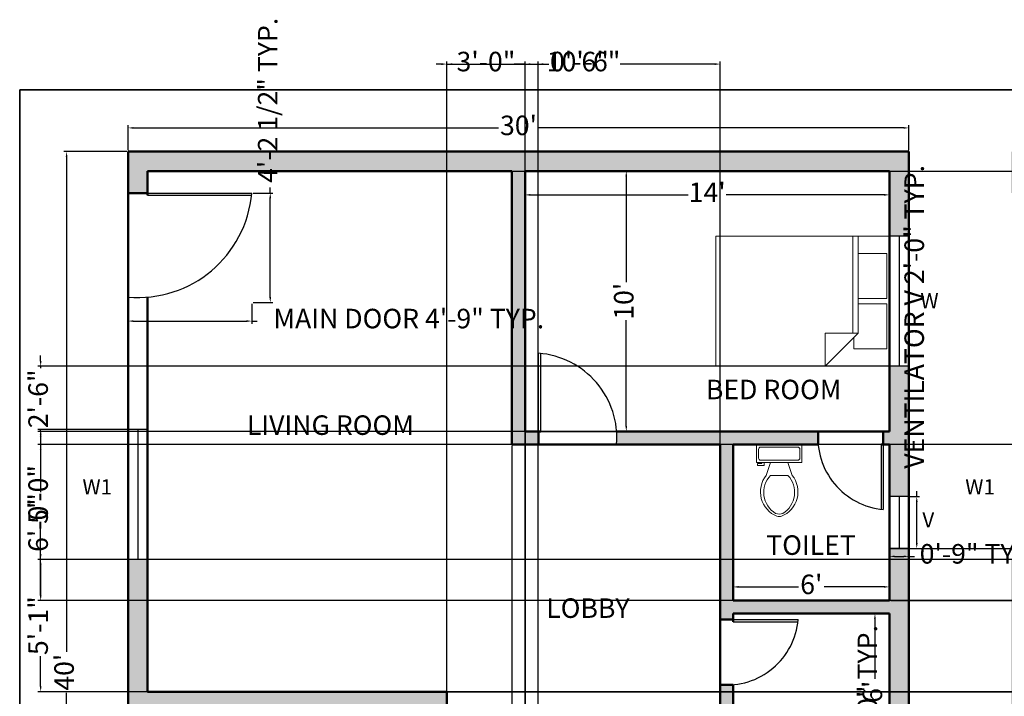
# Model space of a CAD drawing. Units: inches. Extents: x 2463 to 3327, y 6994 to 7582.
# Tile 3 of 5: x 2463 to 2917, y 7270 to 7582. Entities that reach past the tile are written whole.
import ezdxf

# ---------------------------------------------------------------- set-up
doc = ezdxf.new("R2010")
doc.units = ezdxf.units.IN
for name, color, linetype, lineweight in [('A-ANNO-DIMS', 2, 'Continuous', 18), ('A-ANNO-TEXT', 7, 'Continuous', 18), ('A-ANNO-TTLB', 7, 'Continuous', 35), ('A-AREA-IDEN', 3, 'Continuous', 25), ('A-DOOR', 4, 'Continuous', 25), ('A-FLOR-FIXT', 8, 'Continuous', 18), ('A-FURN', 8, 'Continuous', 18), ('A-GLAZ', 4, 'Continuous', 25), ('A-WALL', 7, 'Continuous', 50), ('A-WALL-PATT', 252, 'Continuous', 13)]:
    doc.layers.add(name, color=color, linetype=linetype, lineweight=lineweight)
doc.styles.get("Standard").update_dxf_attribs({"font": 'times.ttf'})
doc.dimstyles.new('ISO-25', dxfattribs={"dimtxt": 9, "dimasz": 2.5, "dimexe": 1.25, "dimexo": 0.625, "dimgap": 2, "dimtad": 0, "dimdec": 1, "dimlunit": 4, "dimtxsty": 'Standard', "dimcen": 2.5, "dimadec": 0, "dimazin": 0, "dimtfac": 1, "dimtdec": 1, "dimtmove": 0, "dimatfit": 3, "dimfxl": 1, "dimarcsym": 0})

# ---------------------------------------------------------------- blocks, each defined once
blk = doc.blocks.new('*D1')
at = {"layer": 'A-ANNO-DIMS', "color": 0, "lineweight": -2, "transparency": 16777216}
for p, q in [((2696.43, 7511.2), (2696.43, 7499.6)), ((2864.43, 7511.2), (2864.43, 7499.6)), ((2698.93, 7500.85), (2771.65, 7500.85)), ((2861.93, 7500.85), (2789.21, 7500.85))]:
    blk.add_line(p, q, dxfattribs=at)
at = {"layer": 'A-ANNO-DIMS', "color": 0, "transparency": 16777216}
for points in [[(2698.93, 7501.27), (2698.93, 7500.43), (2696.43, 7500.85)], [(2861.93, 7501.27), (2861.93, 7500.43), (2864.43, 7500.85)]]:
    blk.add_solid(points, dxfattribs=at)
at = {"layer": 'Defpoints', "color": 0, "transparency": 16777216}
for p in [(2696.43, 7511.83), (2864.43, 7511.83), (2864.43, 7500.85)]:
    blk.add_point(p, dxfattribs=at)
at = {"layer": 'A-ANNO-DIMS', "color": 0, "transparency": 16777216, "insert": (2780.43, 7500.85), "char_height": 9, "attachment_point": 5}
blk.add_mtext("14'", dxfattribs=at)
blk = doc.blocks.new('*D2')
at = {"layer": 'A-ANNO-DIMS', "color": 0, "lineweight": -2, "transparency": 16777216}
for p, q in [((2697.06, 7511.83), (2744.37, 7511.83)), ((2743.12, 7509.33), (2743.12, 7460.61)), ((2743.12, 7394.33), (2743.12, 7443.04)), ((2697.06, 7391.83), (2744.37, 7391.83))]:
    blk.add_line(p, q, dxfattribs=at)
at = {"layer": 'A-ANNO-DIMS', "color": 0, "transparency": 16777216}
for points in [[(2742.7, 7509.33), (2743.53, 7509.33), (2743.12, 7511.83)], [(2742.7, 7394.33), (2743.53, 7394.33), (2743.12, 7391.83)]]:
    blk.add_solid(points, dxfattribs=at)
at = {"layer": 'Defpoints', "color": 0, "transparency": 16777216}
for p in [(2696.43, 7511.83), (2696.43, 7391.83), (2743.12, 7391.83)]:
    blk.add_point(p, dxfattribs=at)
at = {"layer": 'A-ANNO-DIMS', "color": 0, "transparency": 16777216, "insert": (2743.12, 7451.83), "char_height": 9, "attachment_point": 5, "rotation": 90}
blk.add_mtext("10'", dxfattribs=at)
blk = doc.blocks.new('*D3')
at = {"layer": 'A-ANNO-DIMS', "color": 0, "lineweight": -2, "transparency": 16777216}
for p, q in [((2863.81, 7307.83), (2856.5, 7307.83)), ((2857.75, 7305.33), (2857.75, 7277.78)), ((2857.75, 7238.33), (2857.75, 7265.87)), ((2863.81, 7235.83), (2856.5, 7235.83))]:
    blk.add_line(p, q, dxfattribs=at)
at = {"layer": 'A-ANNO-DIMS', "color": 0, "transparency": 16777216}
for points in [[(2857.34, 7305.33), (2858.17, 7305.33), (2857.75, 7307.83)], [(2857.34, 7238.33), (2858.17, 7238.33), (2857.75, 7235.83)]]:
    blk.add_solid(points, dxfattribs=at)
at = {"layer": 'Defpoints', "color": 0, "transparency": 16777216}
for p in [(2857.75, 7307.83), (2864.43, 7307.83), (2864.43, 7235.83)]:
    blk.add_point(p, dxfattribs=at)
at = {"layer": 'A-ANNO-DIMS', "color": 0, "transparency": 16777216, "insert": (2857.75, 7271.83), "char_height": 9, "attachment_point": 5, "rotation": 90}
blk.add_mtext("6'", dxfattribs=at)
blk = doc.blocks.new('Bed - Queen')
for p, q in [((0, -80.00003), (0, 0)), ((0, 0), (59.99999, 0)), ((59.99999, 0), (59.99999, -80.00003)), ((7.99999, -1.2), (28.79998, -1.2)), ((7.99999, -14.4), (7.99999, -1.2)), ((28.79998, -1.2), (28.79998, -14.4)), ((31.19999, -1.2), (51.99999, -1.2)), ((31.19999, -14.4), (31.19999, -1.2)), ((51.99999, -1.2), (51.99999, -16.4)), ((0, -14.4), (44.8, -14.4)), ((44.8, -16.8), (0, -16.8)), ((59.99999, -29.6), (44.8, -14.4)), ((44.8, -14.4), (44.8, -29.6)), ((51.99999, -16.4), (46.79936, -16.4)), ((44.8, -29.6), (59.99999, -29.6)), ((59.99999, -80.00003), (0, -80.00003))]:
    blk.add_line(p, q)
blk = doc.blocks.new('*D13')
at = {"layer": 'A-ANNO-DIMS', "color": 0, "lineweight": -2, "transparency": 16777216}
for p, q in [((2792.43, 7314.45), (2792.43, 7321.4)), ((2794.93, 7320.15), (2822.48, 7320.15)), ((2861.93, 7320.15), (2834.38, 7320.15)), ((2864.43, 7314.45), (2864.43, 7321.4))]:
    blk.add_line(p, q, dxfattribs=at)
at = {"layer": 'A-ANNO-DIMS', "color": 0, "transparency": 16777216}
for points in [[(2794.93, 7320.57), (2794.93, 7319.73), (2792.43, 7320.15)], [(2861.93, 7320.57), (2861.93, 7319.73), (2864.43, 7320.15)]]:
    blk.add_solid(points, dxfattribs=at)
at = {"layer": 'Defpoints', "color": 0, "transparency": 16777216}
for p in [(2864.43, 7320.15), (2792.43, 7313.83), (2864.43, 7313.83)]:
    blk.add_point(p, dxfattribs=at)
at = {"layer": 'A-ANNO-DIMS', "color": 0, "transparency": 16777216, "insert": (2828.43, 7320.15), "char_height": 9, "attachment_point": 5}
blk.add_mtext("6'", dxfattribs=at)
blk = doc.blocks.new('*U11')
for p, q in [((9.5, -6), (9.5, -2)), ((-10, -8.5), (-8, -8.5)), ((-10, -9.5), (-10, -8.5)), ((-8, -8.5), (-8, -8)), ((-7, -8), (-7, -9.5)), ((-4, -8), (-6, -14)), ((4, -8), (6, -14)), ((-7, -9.5), (-10, -9.5)), ((4, -14), (-4, -14))]:
    blk.add_line(p, q)
blk.add_lwpolyline([(10.5, -8), (10.5, 0), (-10.5, 0), (-10.5, -8)], close=True)
for points in [[(-9.5, -2), (-9.5, -6)], [(8.5, -1), (-8.5, -1)], [(-8.5, -7), (8.5, -7)]]:
    blk.add_lwpolyline(points)
for centre, radius, start, end in [((-8.62, -1.88), 0.884, 81.8699, 188.1301), ((8.62, -1.88), 0.884, 351.8699, 98.1301), ((-8.62, -6.12), 0.884, 171.8699, 278.1301), ((8.62, -6.12), 0.884, 261.8699, 8.1301), ((3.52, -21.58), 12.17, 141.4691, 247.9714), ((4.2, -21.82), 11.33, 136.3677, 238.9468), ((-3.52, -21.58), 12.17, 292.0284, 38.5307), ((-4.2, -21.82), 11.33, 301.053, 43.6321), ((0, -27.88), 4, 245.7318, 294.2682), ((0, -29), 4, 254.8605, 285.1395)]:
    blk.add_arc(centre, radius, start, end)
blk = doc.blocks.new('*D24')
at = {"layer": 'A-ANNO-DIMS', "color": 0, "lineweight": -2, "transparency": 16777216}
for p, q in [((2513.43, 7521.45), (2513.43, 7532.96)), ((2515.93, 7531.71), (2684.14, 7531.71)), ((2870.93, 7531.71), (2702.72, 7531.71)), ((2873.43, 7521.45), (2873.43, 7532.96))]:
    blk.add_line(p, q, dxfattribs=at)
at = {"layer": 'A-ANNO-DIMS', "color": 0, "transparency": 16777216}
for points in [[(2515.93, 7532.13), (2515.93, 7531.29), (2513.43, 7531.71)], [(2870.93, 7532.13), (2870.93, 7531.29), (2873.43, 7531.71)]]:
    blk.add_solid(points, dxfattribs=at)
at = {"layer": 'Defpoints', "color": 0, "transparency": 16777216}
for p in [(2873.43, 7531.71), (2513.43, 7520.83), (2873.43, 7520.83)]:
    blk.add_point(p, dxfattribs=at)
at = {"layer": 'A-ANNO-DIMS', "color": 0, "transparency": 16777216, "insert": (2693.43, 7531.71), "char_height": 9, "attachment_point": 5}
blk.add_mtext("30'", dxfattribs=at)
blk = doc.blocks.new('*D26')
at = {"layer": 'A-ANNO-DIMS', "color": 0, "lineweight": -2, "transparency": 16777216}
for p, q in [((2512.81, 7520.83), (2483.85, 7520.83)), ((2485.1, 7518.33), (2485.1, 7290.28)), ((2485.1, 7043.33), (2485.1, 7271.37)), ((2512.81, 7040.83), (2483.85, 7040.83))]:
    blk.add_line(p, q, dxfattribs=at)
at = {"layer": 'A-ANNO-DIMS', "color": 0, "transparency": 16777216}
for points in [[(2484.68, 7518.33), (2485.51, 7518.33), (2485.1, 7520.83)], [(2484.68, 7043.33), (2485.51, 7043.33), (2485.1, 7040.83)]]:
    blk.add_solid(points, dxfattribs=at)
at = {"layer": 'Defpoints', "color": 0, "transparency": 16777216}
for p in [(2513.43, 7520.83), (2485.1, 7040.83), (2513.43, 7040.83)]:
    blk.add_point(p, dxfattribs=at)
at = {"layer": 'A-ANNO-DIMS', "color": 0, "transparency": 16777216, "insert": (2485.1, 7280.83), "char_height": 9, "attachment_point": 5, "rotation": 90}
blk.add_mtext("40'", dxfattribs=at)
blk = doc.blocks.new('DOOR-36')
for p, q in [((0, 6), (0, 42)), ((1, 6), (1, 41.91))]:
    blk.add_line(p, q)
blk.add_arc((-3, 3), 39.12, 355.6013, 85.6013)
blk = doc.blocks.new('DOOR-30')
for p, q in [((29.14, 30), (29.14, 0)), ((30.14, 30), (30.14, 0))]:
    blk.add_line(p, q)
blk.add_arc((33.14, 33), 33.14, 174.8056, 264.8056)
blk = doc.blocks.new('DOOR-48')
for p, q in [((9, 48.19), (57, 48.19)), ((9, 47.19), (56.91, 47.19))]:
    blk.add_line(p, q)
blk.add_arc((4.5, 52.69), 52.69, 265.1009, 355.1009)
blk = doc.blocks.new('WIN-60')
for p, q in [((9, 60), (0, 60)), ((4.5, 60), (4.5, 0)), ((9, 0), (0, 0))]:
    blk.add_line(p, q)
blk = doc.blocks.new('WIN-24')
for p, q in [((9, 24), (0, 24)), ((4.5, 24), (4.5, 0)), ((9, 0), (0, 0))]:
    blk.add_line(p, q)
blk = doc.blocks.new('*D37')
at = {"layer": 'A-ANNO-DIMS', "color": 0, "lineweight": -2, "transparency": 16777216}
for p, q in [((2855.43, 7169.83), (2855.43, 7172.33)), ((2863.81, 7169.83), (2854.18, 7169.83)), ((2855.43, 7112.33), (2855.43, 7167.33)), ((2863.81, 7109.83), (2854.18, 7109.83))]:
    blk.add_line(p, q, dxfattribs=at)
at = {"layer": 'A-ANNO-DIMS', "color": 0, "transparency": 16777216}
for points in [[(2855.01, 7167.33), (2855.85, 7167.33), (2855.43, 7169.83)], [(2855.01, 7112.33), (2855.85, 7112.33), (2855.43, 7109.83)]]:
    blk.add_solid(points, dxfattribs=at)
at = {"layer": 'Defpoints', "color": 0, "transparency": 16777216}
for p in [(2855.43, 7169.83), (2864.43, 7169.83), (2864.43, 7109.83)]:
    blk.add_point(p, dxfattribs=at)
at = {"layer": 'A-ANNO-DIMS', "color": 0, "transparency": 16777216, "insert": (2855.43, 7241.15), "char_height": 9, "attachment_point": 5, "rotation": 90}
blk.add_mtext('WINDOW W 5\'-0" TYP.', dxfattribs=at)
blk = doc.blocks.new('*D39')
at = {"layer": 'A-ANNO-DIMS', "color": 0, "lineweight": -2, "transparency": 16777216}
for p, q in [((2877.03, 7361.83), (2877.03, 7364.33)), ((2874.06, 7361.83), (2878.28, 7361.83)), ((2877.03, 7340.33), (2877.03, 7359.33)), ((2874.06, 7337.83), (2878.28, 7337.83))]:
    blk.add_line(p, q, dxfattribs=at)
at = {"layer": 'A-ANNO-DIMS', "color": 0, "transparency": 16777216}
for points in [[(2876.61, 7359.33), (2877.45, 7359.33), (2877.03, 7361.83)], [(2876.61, 7340.33), (2877.45, 7340.33), (2877.03, 7337.83)]]:
    blk.add_solid(points, dxfattribs=at)
at = {"layer": 'Defpoints', "color": 0, "transparency": 16777216}
for p in [(2873.43, 7361.83), (2877.03, 7361.83), (2873.43, 7337.83)]:
    blk.add_point(p, dxfattribs=at)
at = {"layer": 'A-ANNO-DIMS', "color": 0, "transparency": 16777216, "insert": (2877.03, 7444.63), "char_height": 9, "attachment_point": 5, "rotation": 90}
blk.add_mtext('VENTILATOR V 2\'-0" TYP.', dxfattribs=at)
blk = doc.blocks.new('*D40')
at = {"layer": 'A-ANNO-DIMS', "color": 0, "lineweight": -2, "transparency": 16777216}
for p, q in [((2864.43, 7337.2), (2864.43, 7332.98)), ((2873.43, 7337.2), (2873.43, 7332.98)), ((2866.93, 7334.23), (2870.93, 7334.23)), ((2873.43, 7334.23), (2875.93, 7334.23))]:
    blk.add_line(p, q, dxfattribs=at)
at = {"layer": 'A-ANNO-DIMS', "color": 0, "transparency": 16777216}
for points in [[(2866.93, 7334.64), (2866.93, 7333.81), (2864.43, 7334.23)], [(2870.93, 7334.64), (2870.93, 7333.81), (2873.43, 7334.23)]]:
    blk.add_solid(points, dxfattribs=at)
at = {"layer": 'Defpoints', "color": 0, "transparency": 16777216}
for p in [(2864.43, 7337.83), (2873.43, 7337.83), (2873.43, 7334.23)]:
    blk.add_point(p, dxfattribs=at)
at = {"layer": 'A-ANNO-DIMS', "color": 0, "transparency": 16777216, "insert": (2905.86, 7334.23), "char_height": 9, "attachment_point": 5}
blk.add_mtext('0\'-9" TYP.', dxfattribs=at)
blk = doc.blocks.new('*D47')
at = {"layer": 'A-ANNO-DIMS', "color": 0, "lineweight": -2, "transparency": 16777216}
for p, q in [((2513.43, 7450.6), (2513.43, 7441.42)), ((2570.43, 7450.6), (2570.43, 7441.42)), ((2515.93, 7442.67), (2567.93, 7442.67)), ((2570.43, 7442.67), (2572.93, 7442.67))]:
    blk.add_line(p, q, dxfattribs=at)
at = {"layer": 'A-ANNO-DIMS', "color": 0, "transparency": 16777216}
for points in [[(2515.93, 7443.09), (2515.93, 7442.26), (2513.43, 7442.67)], [(2567.93, 7443.09), (2567.93, 7442.26), (2570.43, 7442.67)]]:
    blk.add_solid(points, dxfattribs=at)
at = {"layer": 'Defpoints', "color": 0, "transparency": 16777216}
for p in [(2513.43, 7451.22), (2570.43, 7451.22), (2570.43, 7442.67)]:
    blk.add_point(p, dxfattribs=at)
at = {"layer": 'A-ANNO-DIMS', "color": 0, "transparency": 16777216, "insert": (2642.86, 7442.67), "char_height": 9, "attachment_point": 5}
blk.add_mtext('MAIN DOOR 4\'-9" TYP.', dxfattribs=at)
blk = doc.blocks.new('*D48')
at = {"layer": 'A-ANNO-DIMS', "color": 0, "lineweight": -2, "transparency": 16777216}
for p, q in [((2578.98, 7501.71), (2578.98, 7504.21)), ((2571.06, 7501.71), (2580.23, 7501.71)), ((2578.98, 7453.72), (2578.98, 7499.21)), ((2571.06, 7451.22), (2580.23, 7451.22))]:
    blk.add_line(p, q, dxfattribs=at)
at = {"layer": 'A-ANNO-DIMS', "color": 0, "transparency": 16777216}
for points in [[(2578.56, 7499.21), (2579.4, 7499.21), (2578.98, 7501.71)], [(2578.56, 7453.72), (2579.4, 7453.72), (2578.98, 7451.22)]]:
    blk.add_solid(points, dxfattribs=at)
at = {"layer": 'Defpoints', "color": 0, "transparency": 16777216}
for p in [(2570.43, 7501.71), (2578.98, 7501.71), (2570.43, 7451.22)]:
    blk.add_point(p, dxfattribs=at)
at = {"layer": 'A-ANNO-DIMS', "color": 0, "transparency": 16777216, "insert": (2578.98, 7544.43), "char_height": 9, "attachment_point": 5, "rotation": 90}
blk.add_mtext('4\'-2 1/2" TYP.', dxfattribs=at)
blk = doc.blocks.new('*D49')
at = {"layer": 'A-ANNO-DIMS', "color": 0, "lineweight": -2, "transparency": 16777216}
for p, q in [((2696.43, 7391.2), (2696.43, 6999.28)), ((2690.43, 7385.2), (2690.43, 6999.28)), ((2687.93, 7000.53), (2685.43, 7000.53)), ((2690.43, 7000.53), (2696.43, 7000.53)), ((2698.93, 7000.53), (2701.43, 7000.53))]:
    blk.add_line(p, q, dxfattribs=at)
at = {"layer": 'A-ANNO-DIMS', "color": 0, "transparency": 16777216}
for points in [[(2687.93, 7000.94), (2687.93, 7000.11), (2690.43, 7000.53)], [(2698.93, 7000.94), (2698.93, 7000.11), (2696.43, 7000.53)]]:
    blk.add_solid(points, dxfattribs=at)
at = {"layer": 'Defpoints', "color": 0, "transparency": 16777216}
for p in [(2696.43, 7391.83), (2690.43, 7385.83), (2696.43, 7000.53)]:
    blk.add_point(p, dxfattribs=at)
at = {"layer": 'A-ANNO-DIMS', "color": 0, "transparency": 16777216, "insert": (2715.52, 7000.53), "char_height": 9, "attachment_point": 5}
blk.add_mtext('0\'-6"', dxfattribs=at)
blk = doc.blocks.new('*D50')
at = {"layer": 'A-ANNO-DIMS', "color": 0, "lineweight": -2, "transparency": 16777216}
for p, q in [((2791.81, 7385.83), (2471.88, 7385.83)), ((2473.13, 7383.33), (2473.13, 7363.87)), ((2473.13, 7316.33), (2473.13, 7335.79)), ((2791.81, 7313.83), (2471.88, 7313.83))]:
    blk.add_line(p, q, dxfattribs=at)
at = {"layer": 'A-ANNO-DIMS', "color": 0, "transparency": 16777216}
for points in [[(2472.71, 7383.33), (2473.55, 7383.33), (2473.13, 7385.83)], [(2472.71, 7316.33), (2473.55, 7316.33), (2473.13, 7313.83)]]:
    blk.add_solid(points, dxfattribs=at)
at = {"layer": 'Defpoints', "color": 0, "transparency": 16777216}
for p in [(2792.43, 7385.83), (2473.13, 7313.83), (2792.43, 7313.83)]:
    blk.add_point(p, dxfattribs=at)
at = {"layer": 'A-ANNO-DIMS', "color": 0, "transparency": 16777216, "insert": (2473.13, 7349.83), "char_height": 9, "attachment_point": 5, "rotation": 90}
blk.add_mtext('6\'-0"', dxfattribs=at)
blk = doc.blocks.new('*D51')
at = {"layer": 'A-ANNO-DIMS', "color": 0, "lineweight": -2, "transparency": 16777216}
for p, q in [((2523.06, 7511.83), (3321.97, 7511.83)), ((3320.72, 7509.33), (3320.72, 7409.33)), ((3320.72, 7274.33), (3320.72, 7374.32)), ((2523.06, 7271.83), (3321.97, 7271.83))]:
    blk.add_line(p, q, dxfattribs=at)
at = {"layer": 'A-ANNO-DIMS', "color": 0, "transparency": 16777216}
for points in [[(3320.31, 7509.33), (3321.14, 7509.33), (3320.72, 7511.83)], [(3320.31, 7274.33), (3321.14, 7274.33), (3320.72, 7271.83)]]:
    blk.add_solid(points, dxfattribs=at)
at = {"layer": 'Defpoints', "color": 0, "transparency": 16777216}
for p in [(2522.43, 7511.83), (2522.43, 7271.83), (3320.72, 7271.83)]:
    blk.add_point(p, dxfattribs=at)
at = {"layer": 'A-ANNO-DIMS', "color": 0, "transparency": 16777216, "insert": (3320.72, 7391.83), "char_height": 9, "attachment_point": 5, "rotation": 90}
blk.add_mtext('20\'-0"', dxfattribs=at)
blk = doc.blocks.new('*D52')
at = {"layer": 'A-ANNO-DIMS', "color": 0, "lineweight": -2, "transparency": 16777216}
for p, q in [((2660.43, 7272.45), (2660.43, 7562.38)), ((2662.93, 7561.13), (2706.56, 7561.13)), ((2783.93, 7561.13), (2740.3, 7561.13)), ((2786.43, 7230.45), (2786.43, 7562.38))]:
    blk.add_line(p, q, dxfattribs=at)
at = {"layer": 'A-ANNO-DIMS', "color": 0, "transparency": 16777216}
for points in [[(2662.93, 7561.54), (2662.93, 7560.71), (2660.43, 7561.13)], [(2783.93, 7561.54), (2783.93, 7560.71), (2786.43, 7561.13)]]:
    blk.add_solid(points, dxfattribs=at)
at = {"layer": 'Defpoints', "color": 0, "transparency": 16777216}
for p in [(2786.43, 7561.13), (2660.43, 7271.83), (2786.43, 7229.83)]:
    blk.add_point(p, dxfattribs=at)
at = {"layer": 'A-ANNO-DIMS', "color": 0, "transparency": 16777216, "insert": (2723.43, 7561.13), "char_height": 9, "attachment_point": 5}
blk.add_mtext('10\'-6"', dxfattribs=at)
blk = doc.blocks.new('*D55')
at = {"layer": 'A-ANNO-DIMS', "color": 0, "lineweight": -2, "transparency": 16777216}
for p, q in [((2657.93, 7561.13), (2655.43, 7561.13)), ((2660.43, 7190.45), (2660.43, 7562.38)), ((2660.43, 7561.13), (2664.38, 7561.13)), ((2696.43, 7561.13), (2692.49, 7561.13)), ((2696.43, 7200.45), (2696.43, 7562.38)), ((2698.93, 7561.13), (2701.43, 7561.13))]:
    blk.add_line(p, q, dxfattribs=at)
at = {"layer": 'A-ANNO-DIMS', "color": 0, "transparency": 16777216}
for points in [[(2657.93, 7561.54), (2657.93, 7560.71), (2660.43, 7561.13)], [(2698.93, 7561.54), (2698.93, 7560.71), (2696.43, 7561.13)]]:
    blk.add_solid(points, dxfattribs=at)
at = {"layer": 'Defpoints', "color": 0, "transparency": 16777216}
for p in [(2696.43, 7561.13), (2696.43, 7199.83), (2660.43, 7189.83)]:
    blk.add_point(p, dxfattribs=at)
at = {"layer": 'A-ANNO-DIMS', "color": 0, "transparency": 16777216, "insert": (2678.43, 7561.13), "char_height": 9, "attachment_point": 5}
blk.add_mtext('3\'-0"', dxfattribs=at)
blk = doc.blocks.new('*D56')
at = {"layer": 'A-ANNO-DIMS', "color": 0, "lineweight": -2, "transparency": 16777216}
for p, q in [((2693.93, 7561.13), (2691.43, 7561.13)), ((2696.43, 7200.45), (2696.43, 7562.38)), ((2696.43, 7561.13), (2702.43, 7561.13)), ((2702.43, 7200.45), (2702.43, 7562.38)), ((2704.93, 7561.13), (2707.43, 7561.13))]:
    blk.add_line(p, q, dxfattribs=at)
at = {"layer": 'A-ANNO-DIMS', "color": 0, "transparency": 16777216}
for points in [[(2693.93, 7561.54), (2693.93, 7560.71), (2696.43, 7561.13)], [(2704.93, 7561.54), (2704.93, 7560.71), (2702.43, 7561.13)]]:
    blk.add_solid(points, dxfattribs=at)
at = {"layer": 'Defpoints', "color": 0, "transparency": 16777216}
for p in [(2702.43, 7561.13), (2696.43, 7199.83), (2702.43, 7199.83)]:
    blk.add_point(p, dxfattribs=at)
at = {"layer": 'A-ANNO-DIMS', "color": 0, "transparency": 16777216, "insert": (2721.52, 7561.13), "char_height": 9, "attachment_point": 5}
blk.add_mtext('0\'-6"', dxfattribs=at)
blk = doc.blocks.new('*D62')
at = {"layer": 'A-ANNO-DIMS', "color": 0, "lineweight": -2, "transparency": 16777216}
for p, q in [((2521.81, 7332.77), (2471.88, 7332.77)), ((2473.13, 7330.27), (2473.13, 7316.3)), ((2473.13, 7274.33), (2473.13, 7288.29)), ((2521.81, 7271.83), (2471.88, 7271.83))]:
    blk.add_line(p, q, dxfattribs=at)
at = {"layer": 'A-ANNO-DIMS', "color": 0, "transparency": 16777216}
for points in [[(2472.71, 7330.27), (2473.55, 7330.27), (2473.13, 7332.77)], [(2472.71, 7274.33), (2473.55, 7274.33), (2473.13, 7271.83)]]:
    blk.add_solid(points, dxfattribs=at)
at = {"layer": 'Defpoints', "color": 0, "transparency": 16777216}
for p in [(2473.13, 7332.77), (2522.43, 7332.77), (2522.43, 7271.83)]:
    blk.add_point(p, dxfattribs=at)
at = {"layer": 'A-ANNO-DIMS', "color": 0, "transparency": 16777216, "insert": (2473.13, 7302.3), "char_height": 9, "attachment_point": 5, "rotation": 90}
blk.add_mtext('5\'-1"', dxfattribs=at)
blk = doc.blocks.new('*D63')
at = {"layer": 'A-ANNO-DIMS', "color": 0, "lineweight": -2, "transparency": 16777216}
for p, q in [((2512.81, 7392.77), (2471.88, 7392.77)), ((2473.13, 7390.27), (2473.13, 7376.77)), ((2473.13, 7335.27), (2473.13, 7348.76)), ((2512.81, 7332.77), (2471.88, 7332.77))]:
    blk.add_line(p, q, dxfattribs=at)
at = {"layer": 'A-ANNO-DIMS', "color": 0, "transparency": 16777216}
for points in [[(2472.71, 7390.27), (2473.55, 7390.27), (2473.13, 7392.77)], [(2472.71, 7335.27), (2473.55, 7335.27), (2473.13, 7332.77)]]:
    blk.add_solid(points, dxfattribs=at)
at = {"layer": 'Defpoints', "color": 0, "transparency": 16777216}
for p in [(2473.13, 7392.77), (2513.43, 7392.77), (2513.43, 7332.77)]:
    blk.add_point(p, dxfattribs=at)
at = {"layer": 'A-ANNO-DIMS', "color": 0, "transparency": 16777216, "insert": (2473.13, 7362.77), "char_height": 9, "attachment_point": 5, "rotation": 90}
blk.add_mtext('5\'-0"', dxfattribs=at)
blk = doc.blocks.new('*D64')
at = {"layer": 'A-ANNO-DIMS', "color": 0, "lineweight": -2, "transparency": 16777216}
for p, q in [((2473.13, 7424.33), (2473.13, 7426.83)), ((2863.81, 7421.83), (2471.88, 7421.83)), ((2473.13, 7421.83), (2473.13, 7421.01)), ((2863.81, 7391.83), (2471.88, 7391.83)), ((2473.13, 7391.83), (2473.13, 7392.64)), ((2473.13, 7389.33), (2473.13, 7386.83))]:
    blk.add_line(p, q, dxfattribs=at)
at = {"layer": 'A-ANNO-DIMS', "color": 0, "transparency": 16777216}
for points in [[(2472.71, 7424.33), (2473.55, 7424.33), (2473.13, 7421.83)], [(2472.71, 7389.33), (2473.55, 7389.33), (2473.13, 7391.83)]]:
    blk.add_solid(points, dxfattribs=at)
at = {"layer": 'Defpoints', "color": 0, "transparency": 16777216}
for p in [(2473.13, 7421.83), (2864.43, 7421.83), (2864.43, 7391.83)]:
    blk.add_point(p, dxfattribs=at)
at = {"layer": 'A-ANNO-DIMS', "color": 0, "transparency": 16777216, "insert": (2473.13, 7406.83), "char_height": 9, "attachment_point": 5, "rotation": 90}
blk.add_mtext('2\'-6"', dxfattribs=at)
blk = doc.blocks.new('*D65')
at = {"layer": 'A-ANNO-DIMS', "color": 0, "lineweight": -2, "transparency": 16777216}
for p, q in [((3320.72, 7337.83), (3320.72, 7340.33)), ((2865.06, 7337.83), (3321.97, 7337.83)), ((3320.72, 7316.33), (3320.72, 7335.33)), ((2865.06, 7313.83), (3321.97, 7313.83))]:
    blk.add_line(p, q, dxfattribs=at)
at = {"layer": 'A-ANNO-DIMS', "color": 0, "transparency": 16777216}
for points in [[(3320.31, 7335.33), (3321.14, 7335.33), (3320.72, 7337.83)], [(3320.31, 7316.33), (3321.14, 7316.33), (3320.72, 7313.83)]]:
    blk.add_solid(points, dxfattribs=at)
at = {"layer": 'Defpoints', "color": 0, "transparency": 16777216}
for p in [(2864.43, 7337.83), (3320.72, 7337.83), (2864.43, 7313.83)]:
    blk.add_point(p, dxfattribs=at)
at = {"layer": 'A-ANNO-DIMS', "color": 0, "transparency": 16777216, "insert": (3320.72, 7354.51), "char_height": 9, "attachment_point": 5, "rotation": 90}
blk.add_mtext('2\'-0"', dxfattribs=at)
blk = doc.blocks.new('*D69')
at = {"layer": 'A-ANNO-DIMS', "color": 0, "lineweight": -2, "transparency": 16777216}
for p, q in [((3198.8, 7385.83), (2471.88, 7385.83)), ((2473.13, 7383.33), (2473.13, 7363.87)), ((2473.13, 7316.33), (2473.13, 7335.79)), ((3198.8, 7313.83), (2471.88, 7313.83))]:
    blk.add_line(p, q, dxfattribs=at)
at = {"layer": 'A-ANNO-DIMS', "color": 0, "transparency": 16777216}
for points in [[(2472.71, 7383.33), (2473.55, 7383.33), (2473.13, 7385.83)], [(2472.71, 7316.33), (2473.55, 7316.33), (2473.13, 7313.83)]]:
    blk.add_solid(points, dxfattribs=at)
at = {"layer": 'Defpoints', "color": 0, "transparency": 16777216}
for p in [(3199.42, 7385.83), (2473.13, 7313.83), (3199.42, 7313.83)]:
    blk.add_point(p, dxfattribs=at)
at = {"layer": 'A-ANNO-DIMS', "color": 0, "transparency": 16777216, "insert": (2473.13, 7349.83), "char_height": 9, "attachment_point": 5, "rotation": 90}
blk.add_mtext('6\'-0"', dxfattribs=at)
blk = doc.blocks.new('*D78')
at = {"layer": 'A-ANNO-DIMS', "color": 0, "lineweight": -2, "transparency": 16777216}
for p, q in [((2928.8, 7332.77), (2471.88, 7332.77)), ((2473.13, 7330.27), (2473.13, 7316.3)), ((2473.13, 7274.33), (2473.13, 7288.29)), ((2928.8, 7271.83), (2471.88, 7271.83))]:
    blk.add_line(p, q, dxfattribs=at)
at = {"layer": 'A-ANNO-DIMS', "color": 0, "transparency": 16777216}
for points in [[(2472.71, 7330.27), (2473.55, 7330.27), (2473.13, 7332.77)], [(2472.71, 7274.33), (2473.55, 7274.33), (2473.13, 7271.83)]]:
    blk.add_solid(points, dxfattribs=at)
at = {"layer": 'Defpoints', "color": 0, "transparency": 16777216}
for p in [(2473.13, 7332.77), (2929.42, 7332.77), (2929.42, 7271.83)]:
    blk.add_point(p, dxfattribs=at)
at = {"layer": 'A-ANNO-DIMS', "color": 0, "transparency": 16777216, "insert": (2473.13, 7302.3), "char_height": 9, "attachment_point": 5, "rotation": 90}
blk.add_mtext('5\'-1"', dxfattribs=at)

msp = doc.modelspace()

# ---------------------------------------------------------------- hatches: boundary and pattern name
at = {"layer": 'A-WALL-PATT'}
h = msp.add_hatch(color=256, dxfattribs=at)
h.dxf.hatch_style = 1
h.paths.add_polyline_path([(2522.43, 7511.83), (2690.43, 7511.83), (2690.43, 7385.83), (2696.43, 7385.83), (2702.68, 7385.83), (2702.68, 7391.83), (2696.43, 7391.83), (2696.43, 7511.83), (2864.43, 7511.83), (2864.43, 7481.83), (2873.43, 7481.83), (2873.43, 7520.83), (2513.43, 7520.83), (2513.43, 7501.71), (2522.43, 7501.71)])
h.paths.add_polyline_path([(2522.43, 7453.71, -0.042779), (2513.43, 7453.71), (2513.43, 7392.77), (2522.43, 7392.77)], flags=0)
h.paths.add_polyline_path([(2522.43, 7332.77), (2513.43, 7332.77), (2513.43, 7226.83), (2522.43, 7226.83), (2522.43, 7265.83), (2654.43, 7265.83), (2654.43, 7263.42), (2660.43, 7263.42), (2660.43, 7271.83), (2522.43, 7271.83)])
h.paths.add_polyline_path([(2873.43, 7421.83), (2864.43, 7421.83), (2864.43, 7391.83), (2861.59, 7391.83), (2861.59, 7385.83), (2864.43, 7385.83), (2864.43, 7361.83), (2873.43, 7361.83)])
h.paths.add_polyline_path([(2792.43, 7385.83), (2831.59, 7385.83, -0.045361), (2831.59, 7391.83), (2738.68, 7391.83, -0.038405), (2738.68, 7385.83), (2786.43, 7385.83), (2786.43, 7313.83), (2786.43, 7307.83), (2786.43, 7305.07), (2792.43, 7305.07), (2792.43, 7307.83), (2864.43, 7307.83), (2864.43, 7235.83), (2792.43, 7235.83), (2792.43, 7275.07, -0.045361), (2786.43, 7275.07), (2786.43, 7235.83), (2786.43, 7229.83), (2864.43, 7229.83), (2864.43, 7169.83), (2873.43, 7169.83), (2873.43, 7337.83), (2864.43, 7337.83), (2864.43, 7313.83), (2792.43, 7313.83)])
h.paths.add_polyline_path([(2873.43, 7109.83), (2864.43, 7109.83), (2864.43, 7049.83), (2834.43, 7049.83), (2834.43, 7040.83), (2873.43, 7040.83)])
h.paths.add_polyline_path([(2774.43, 7049.83), (2744.43, 7049.83), (2744.43, 7199.83), (2738.43, 7199.83), (2738.43, 7049.83), (2723.43, 7049.83), (2723.43, 7040.83), (2774.43, 7040.83)])
h.paths.add_polyline_path([(2675.43, 7049.83), (2660.43, 7049.83), (2660.43, 7121.83), (2660.43, 7127.83), (2660.43, 7227.42, -0.038405), (2654.43, 7227.42), (2654.43, 7127.83), (2651.08, 7127.83), (2651.08, 7121.83), (2654.43, 7121.83), (2654.43, 7049.83), (2522.43, 7049.83), (2522.43, 7073.83), (2513.43, 7073.83), (2513.43, 7040.83), (2675.43, 7040.83)])
h.paths.add_polyline_path([(2621.08, 7127.83), (2522.43, 7127.83), (2522.43, 7166.83), (2513.43, 7166.83), (2513.43, 7097.83), (2522.43, 7097.83), (2522.43, 7121.83), (2621.08, 7121.83, -0.045361)], flags=17)
h.paths.add_polyline_path([(3280.42, 7520.83), (2920.42, 7520.83), (2920.42, 7501.71), (2929.42, 7501.71), (2929.42, 7511.83), (3097.42, 7511.83), (3097.42, 7385.83), (3103.42, 7385.83), (3109.67, 7385.83), (3109.67, 7391.83), (3103.42, 7391.83), (3103.42, 7511.83), (3271.42, 7511.83), (3271.42, 7481.83), (3280.42, 7481.83)])
h.paths.add_polyline_path([(3280.42, 7421.83), (3271.42, 7421.83), (3271.42, 7391.83), (3268.58, 7391.83), (3268.58, 7385.83), (3271.42, 7385.83), (3271.42, 7361.83), (3280.42, 7361.83)])
h.paths.add_polyline_path([(3238.58, 7391.83), (3145.67, 7391.83, -0.038405), (3145.67, 7385.83), (3193.42, 7385.83), (3193.42, 7313.83), (3193.42, 7307.83), (3193.42, 7305.07), (3199.42, 7305.07), (3199.42, 7307.83), (3271.42, 7307.83), (3271.42, 7235.83), (3199.42, 7235.83), (3193.42, 7235.83), (3193.42, 7229.83), (3271.42, 7229.83), (3280.42, 7229.83), (3280.42, 7337.83), (3271.42, 7337.83), (3271.42, 7313.83), (3199.42, 7313.83), (3199.42, 7385.83), (3238.58, 7385.83, -0.045361)])
h.paths.add_polyline_path([(3199.42, 7275.07, -0.045361), (3193.42, 7275.07), (3193.42, 7235.83), (3199.42, 7235.83)], flags=17)
h.paths.add_polyline_path([(3193.42, 7235.83), (3145.42, 7235.83), (3145.42, 7227.44), (3151.42, 7227.44), (3151.42, 7229.83), (3193.42, 7229.83)])
h.paths.add_polyline_path([(3151.42, 7199.83, -0.044871), (3145.42, 7199.83), (3145.42, 7049.83), (3130.42, 7049.83), (3130.42, 7040.83), (3151.42, 7040.83), (3151.42, 7049.83)])
h.paths.add_polyline_path([(3082.42, 7049.83), (3067.42, 7049.83), (3067.42, 7121.83), (3067.42, 7127.83), (3067.42, 7227.42, -0.038405), (3061.42, 7227.42), (3061.42, 7127.83), (3058.07, 7127.83), (3058.07, 7121.83), (3061.42, 7121.83), (3061.42, 7049.83), (2929.42, 7049.83), (2929.42, 7073.83), (2920.42, 7073.83), (2920.42, 7040.83), (3082.42, 7040.83)])
h.paths.add_polyline_path([(3028.07, 7121.83), (2997.56, 7121.83), (2997.56, 7113.83), (2991.06, 7113.83), (2993.06, 7107.83, -0.501323), (2988.1, 7088.96, -0.132891), (2986.01, 7088.96, -0.501317), (2981.06, 7107.83), (2983.06, 7113.83), (2980.06, 7113.83), (2980.06, 7112.33), (2977.06, 7112.33), (2977.06, 7113.83), (2976.56, 7113.83), (2976.56, 7121.83), (2929.42, 7121.83), (2929.42, 7097.83), (2920.42, 7097.83), (2920.42, 7166.83), (2929.42, 7166.83), (2929.42, 7127.83), (3028.07, 7127.83, 0.045361)], flags=17)
h.paths.add_polyline_path([(2995.56, 7120.83, -0.414214), (2996.56, 7120.08), (2996.56, 7115.83, -0.414214), (2995.81, 7114.83), (2978.56, 7114.83, -0.414214), (2977.56, 7115.58), (2977.56, 7119.83, -0.414214), (2978.31, 7120.83)], flags=16)
h.paths.add_polyline_path([(2988.7, 7090.3, -0.215004), (2985.41, 7090.3, -0.48008), (2983.06, 7107.83), (2991.06, 7107.83, -0.48008)], flags=16)
h.paths.add_polyline_path([(2929.42, 7265.83), (3061.42, 7265.83), (3061.42, 7263.42), (3067.42, 7263.42), (3067.42, 7271.83), (2929.42, 7271.83), (2929.42, 7332.77), (2920.42, 7332.77), (2920.42, 7226.83), (2929.42, 7226.83)])
h.paths.add_polyline_path([(2929.42, 7453.71, -0.042779), (2920.42, 7453.71), (2920.42, 7392.77), (2929.42, 7392.77)], flags=0)

# ---------------------------------------------------------------- linework, layer by layer
at = {"layer": 'A-ANNO-TTLB'}
msp.add_lwpolyline([(2463.47, 7549.29), (3297.67, 7549.29), (3297.67, 7021.48), (2463.47, 7021.48)], close=True, dxfattribs=at)
at = {"layer": 'A-WALL'}
for p, q in [((2513.43, 7520.83), (2873.43, 7520.83)), ((2513.43, 7040.83), (2513.43, 7520.83)), ((2873.43, 7520.83), (2873.43, 7040.83)), ((2522.43, 7511.83), (2690.43, 7511.83)), ((2522.43, 7501.71), (2522.43, 7511.83)), ((2690.43, 7511.83), (2690.43, 7385.83)), ((2696.43, 7511.83), (2696.43, 7391.83)), ((2696.43, 7511.83), (2864.43, 7511.83)), ((2864.43, 7511.83), (2864.43, 7391.83)), ((2522.43, 7501.71), (2513.43, 7501.71)), ((2522.43, 7500.71), (2522.43, 7501.71)), ((2522.43, 7271.83), (2522.43, 7453.71)), ((2696.43, 7391.83), (2703.68, 7391.83)), ((2702.68, 7391.83), (2702.68, 7385.83)), ((2738.68, 7391.83), (2864.43, 7391.83)), ((2831.59, 7385.83), (2831.59, 7391.83)), ((2861.59, 7385.83), (2861.59, 7391.83)), ((2696.43, 7385.83), (2690.43, 7385.83)), ((2696.43, 7385.83), (2786.43, 7385.83)), ((2786.43, 7385.83), (2786.43, 7313.83)), ((2792.43, 7385.83), (2792.43, 7313.83)), ((2792.43, 7385.83), (2831.59, 7385.83)), ((2860.59, 7385.83), (2864.43, 7385.83)), ((2864.43, 7385.83), (2864.43, 7313.83)), ((2786.43, 7313.83), (2786.43, 7307.83)), ((2792.43, 7313.83), (2864.43, 7313.83)), ((2786.43, 7307.83), (2786.43, 7235.83)), ((2792.43, 7305.07), (2786.43, 7305.07)), ((2792.43, 7307.83), (2864.43, 7307.83)), ((2792.43, 7307.83), (2792.43, 7304.07)), ((2864.43, 7307.83), (2864.43, 7235.83)), ((2792.43, 7275.07), (2786.43, 7275.07)), ((2792.43, 7275.07), (2792.43, 7235.83)), ((2660.43, 7271.83), (2522.43, 7271.83)), ((2660.43, 7127.83), (2660.43, 7271.83))]:
    msp.add_line(p, q, dxfattribs=at)

# ---------------------------------------------------------------- block references
at = {"layer": 'A-DOOR'}
for name, p in [('DOOR-48', (2513.43, 7453.52)), ('DOOR-36', (2702.68, 7385.83)), ('DOOR-30', (2831.45, 7355.83))]:
    msp.add_blockref(name, p, dxfattribs=at)
at = {"layer": 'A-DOOR', "rotation": 90.023010632294}
msp.add_blockref('DOOR-30', (2822.43, 7274.94), dxfattribs=at)
at = {"layer": 'A-FLOR-FIXT'}
msp.add_blockref('*U11', (2813.62, 7385.55), dxfattribs=at)
at = {"layer": 'A-FURN', "rotation": 270}
msp.add_blockref('Bed - Queen', (2864.43, 7481.83), dxfattribs=at)
at = {"layer": 'A-GLAZ'}
for name, p in [('WIN-60', (2864.43, 7421.83)), ('WIN-60', (2513.43, 7332.77)), ('WIN-24', (2864.43, 7337.83))]:
    msp.add_blockref(name, p, dxfattribs=at)

# ---------------------------------------------------------------- texts
at = {"layer": 'A-ANNO-TEXT', "char_height": 7, "attachment_point": 1}
for s, insert in [('\\pxqc;{\\fTimes New Roman|b1|i0|c0|p18;W}', (2868.71, 7455.56)), ('\\pxqc;{\\fTimes New Roman|b1|i0|c0|p18;W1}', (2485.05, 7369.77)), ('\\pxqc;{\\fTimes New Roman|b1|i0|c0|p18;W1}', (2892.04, 7369.77)), ('\\pxqc;{\\fTimes New Roman|b1|i0|c0|p18;V}', (2868.16, 7354.57))]:
    msp.add_mtext_dynamic_manual_height_columns(s, width=28.3852, gutter_width=12.5, heights=[0], dxfattribs=dict(at, insert=insert))
at = {"layer": 'A-AREA-IDEN', "char_height": 9, "attachment_point": 1}
for s, width, insert in [('\\pxqc;{\\fTimes New Roman|b1|i0|c0|p18;BED ROOM}', 86.127, (2768.01, 7415.64)), ('\\pxqc;{\\fTimes New Roman|b1|i0|c0|p18;LIVING ROOM}', 122.533, (2545.43, 7399.21)), ('\\pxqc;{\\fTimes New Roman|b1|i0|c0|p18;TOILET}', 62.7452, (2796.93, 7343.91)), ('\\pxqc;{\\fTimes New Roman|b1|i0|c0|p18;LOBBY}', 90.7623, (2680.05, 7314.86))]:
    msp.add_mtext_dynamic_manual_height_columns(s, width=width, gutter_width=12.5, heights=[0], dxfattribs=dict(at, insert=insert))

# ---------------------------------------------------------------- dimensions: what is measured, and where the dimension line sits
at = {"layer": 'A-ANNO-DIMS'}
for base, p1, p2, text, picture, middle in [((2578.98, 7501.71), (2570.43, 7451.22), (2570.43, 7501.71), '<> TYP.', '*D48', (2578.98, 7544.43)), ((2877.03, 7361.83), (2873.43, 7337.83), (2873.43, 7361.83), 'VENTILATOR V <> TYP.', '*D39', (2877.03, 7444.63)), ((2855.43, 7169.83), (2864.43, 7109.83), (2864.43, 7169.83), 'WINDOW W <> TYP.', '*D37', (2855.43, 7241.15))]:
    dim = msp.add_linear_dim(base=base, p1=p1, p2=p2, angle=90, text=text, dimstyle='ISO-25', override={"dimdec": 1, "dimrnd": 0, "dimzin": 1, "dimlunit": 4, "dimfrac": 2}, dxfattribs=at)
    dim.commit()
    dim.dimension.update_dxf_attribs({"geometry": picture, "text_midpoint": middle})
for base, p1, p2, override, picture, middle in [((2696.43, 7561.13), (2660.43, 7189.83), (2696.43, 7199.83), {"dimdec": 1, "dimlfac": 1, "dimrnd": 0, "dimzin": 1, "dimdsep": 46, "dimlunit": 4, "dimfrac": 2}, '*D55', (2678.43, 7561.13)), ((2786.43, 7561.13), (2660.43, 7271.83), (2786.43, 7229.83), {"dimdec": 1, "dimlfac": 1, "dimrnd": 0, "dimzin": 1, "dimdsep": 46, "dimlunit": 4, "dimfrac": 2}, '*D52', (2723.43, 7561.13)), ((2702.43, 7561.13), (2696.43, 7199.83), (2702.43, 7199.83), {"dimdec": 1, "dimlfac": 1, "dimrnd": 0, "dimzin": 1, "dimdsep": 46, "dimlunit": 4, "dimfrac": 2}, '*D56', (2721.52, 7561.13)), ((2873.43, 7531.71), (2513.43, 7520.83), (2873.43, 7520.83), {"dimclrd": 0, "dimclre": 0, "dimclrt": 0}, '*D24', (2693.43, 7531.71)), ((2864.43, 7500.85), (2696.43, 7511.83), (2864.43, 7511.83), {"dimclrd": 0, "dimclre": 0, "dimclrt": 0}, '*D1', (2780.43, 7500.85)), ((2696.43, 7000.53), (2690.43, 7385.83), (2696.43, 7391.83), {"dimdec": 1, "dimlfac": 1, "dimrnd": 0, "dimzin": 1, "dimdsep": 46, "dimlunit": 4, "dimfrac": 2}, '*D49', (2715.52, 7000.53)), ((2864.43, 7320.15), (2792.43, 7313.83), (2864.43, 7313.83), {"dimclrd": 0, "dimclre": 0, "dimclrt": 0}, '*D13', (2828.43, 7320.15))]:
    dim = msp.add_linear_dim(base=base, p1=p1, p2=p2, dimstyle='ISO-25', override=override, dxfattribs=at)
    dim.commit()
    dim.dimension.update_dxf_attribs({"geometry": picture, "text_midpoint": middle})
for base, p1, p2, override, picture, middle in [((2485.1, 7040.83), (2513.43, 7520.83), (2513.43, 7040.83), {"dimclrd": 0, "dimclre": 0, "dimclrt": 0}, '*D26', (2485.1, 7280.83)), ((3320.72, 7271.83), (2522.43, 7511.83), (2522.43, 7271.83), {"dimdec": 1, "dimlfac": 1, "dimrnd": 0, "dimzin": 1, "dimdsep": 46, "dimlunit": 4, "dimfrac": 2}, '*D51', (3320.72, 7391.83)), ((2743.12, 7391.83), (2696.43, 7511.83), (2696.43, 7391.83), {"dimclrd": 0, "dimclre": 0, "dimclrt": 0}, '*D2', (2743.12, 7451.83)), ((2473.13, 7421.83), (2864.43, 7391.83), (2864.43, 7421.83), {"dimdec": 1, "dimlfac": 1, "dimrnd": 0, "dimzin": 1, "dimdsep": 46, "dimlunit": 4, "dimfrac": 2}, '*D64', (2473.13, 7406.83)), ((2473.13, 7392.77), (2513.43, 7332.77), (2513.43, 7392.77), {"dimdec": 1, "dimlfac": 1, "dimrnd": 0, "dimzin": 1, "dimdsep": 46, "dimlunit": 4, "dimfrac": 2}, '*D63', (2473.13, 7362.77)), ((2473.13, 7313.83), (2792.43, 7385.83), (2792.43, 7313.83), {"dimdec": 1, "dimlfac": 1, "dimrnd": 0, "dimzin": 1, "dimdsep": 46, "dimlunit": 4, "dimfrac": 2}, '*D50', (2473.13, 7349.83)), ((2473.13, 7313.83), (3199.42, 7385.83), (3199.42, 7313.83), {"dimdec": 1, "dimlfac": 1, "dimrnd": 0, "dimzin": 1, "dimdsep": 46, "dimlunit": 4, "dimfrac": 2}, '*D69', (2473.13, 7349.83)), ((3320.72, 7337.83), (2864.43, 7313.83), (2864.43, 7337.83), {"dimdec": 1, "dimlfac": 1, "dimrnd": 0, "dimzin": 1, "dimdsep": 46, "dimlunit": 4, "dimfrac": 2}, '*D65', (3320.72, 7354.51)), ((2473.13, 7332.77), (2522.43, 7271.83), (2522.43, 7332.77), {"dimdec": 1, "dimlfac": 1, "dimrnd": 0, "dimzin": 1, "dimdsep": 46, "dimlunit": 4, "dimfrac": 2}, '*D62', (2473.13, 7302.3)), ((2473.13, 7332.77), (2929.42, 7271.83), (2929.42, 7332.77), {"dimdec": 1, "dimlfac": 1, "dimrnd": 0, "dimzin": 1, "dimdsep": 46, "dimlunit": 4, "dimfrac": 2}, '*D78', (2473.13, 7302.3)), ((2857.75, 7307.83), (2864.43, 7235.83), (2864.43, 7307.83), {"dimclrd": 0, "dimclre": 0, "dimclrt": 0}, '*D3', (2857.75, 7271.83))]:
    dim = msp.add_linear_dim(base=base, p1=p1, p2=p2, angle=90, dimstyle='ISO-25', override=override, dxfattribs=at)
    dim.commit()
    dim.dimension.update_dxf_attribs({"geometry": picture, "text_midpoint": middle})
for base, p1, p2, text, picture, middle in [((2570.43, 7442.67), (2513.43, 7451.22), (2570.43, 7451.22), 'MAIN DOOR <> TYP.', '*D47', (2642.86, 7442.67)), ((2873.43, 7334.23), (2864.43, 7337.83), (2873.43, 7337.83), '<> TYP.', '*D40', (2905.86, 7334.23))]:
    dim = msp.add_linear_dim(base=base, p1=p1, p2=p2, text=text, dimstyle='ISO-25', override={"dimdec": 1, "dimrnd": 0, "dimzin": 1, "dimlunit": 4, "dimfrac": 2}, dxfattribs=at)
    dim.commit()
    dim.dimension.update_dxf_attribs({"geometry": picture, "text_midpoint": middle})

doc.saveas('drawing.dxf')
